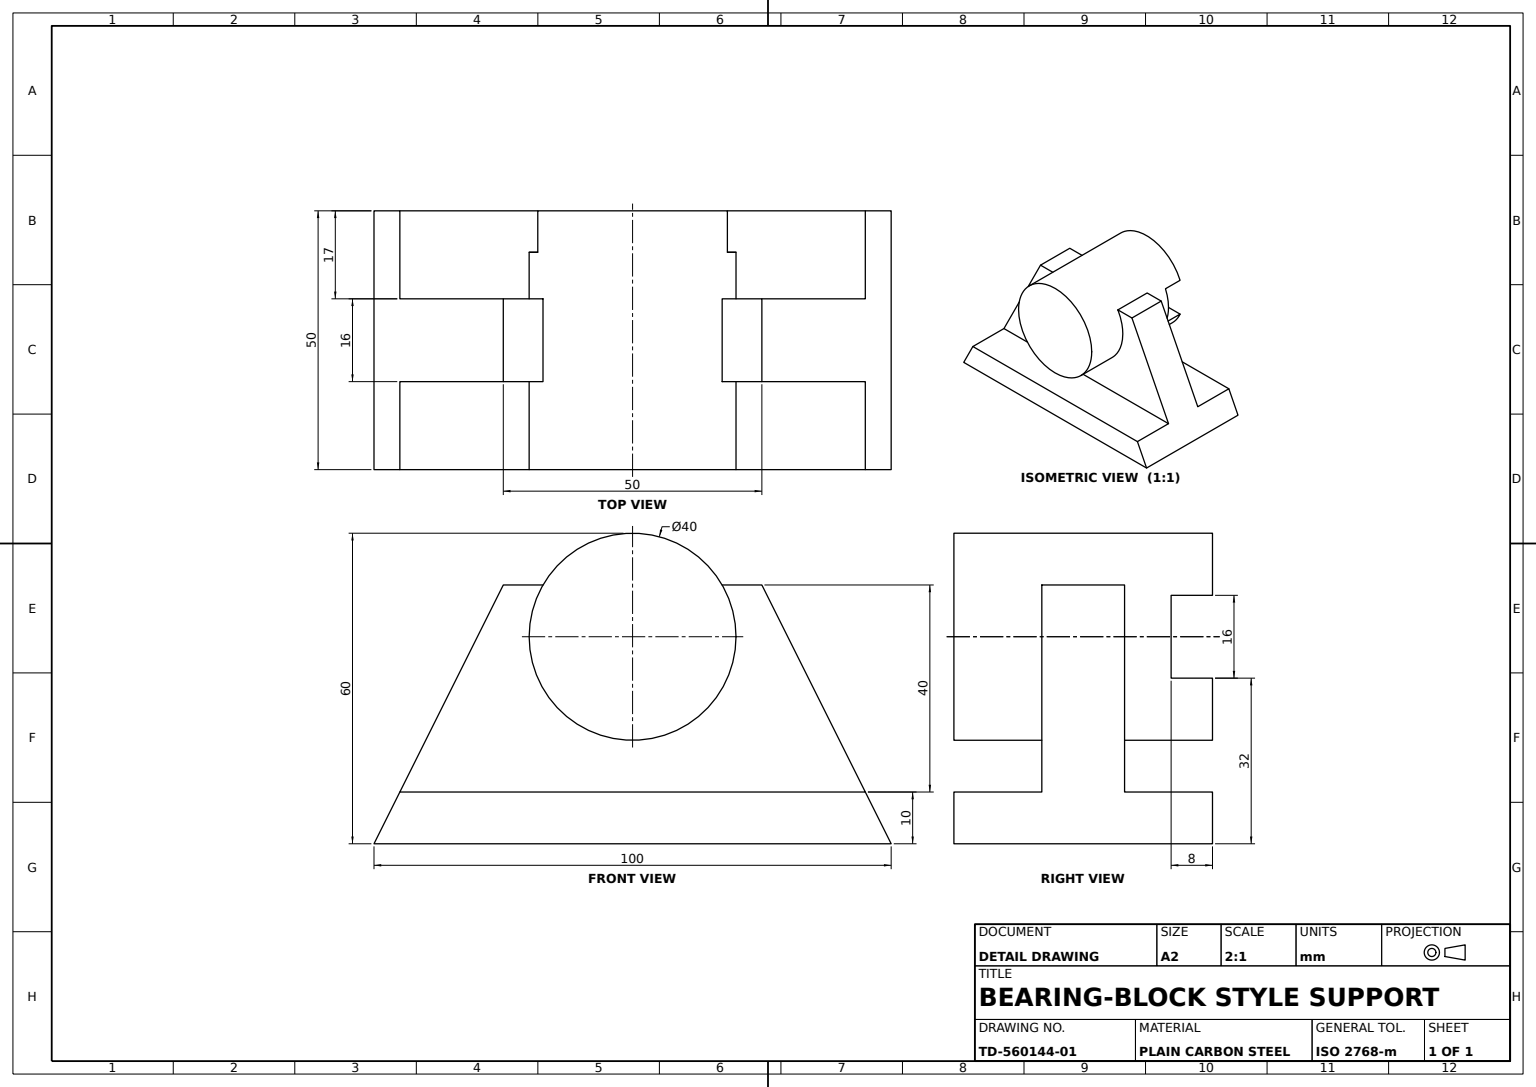
from build123d import *

# Parameters (mm, degrees)
BASE_PLATE_DEPTH        = 25
SUPPORT_UPRIGHT_DEPTH   = 8
SHAFT_CYLINDER_SKETCH_R = 20
SHAFT_CYLINDER_40_DEPTH = 25
SHAFT_START             = -8
SHAFT_END_NOTCH_DEPTH   = 8


with BuildPart() as part:
    # Base Plate Sketch → Base Plate (new, symmetric)
    with BuildSketch(Plane.XY):
        Polygon((0, 0), (100, 0), (95, 10), (5, 10), align=None)
    extrude(amount=BASE_PLATE_DEPTH, both=True)

    # Support Upright Sketch → Support Upright (add, symmetric)
    with BuildSketch(Plane.XY):
        Polygon((5, 10), (95, 10), (75, 50), (25, 50), align=None)
    extrude(amount=SUPPORT_UPRIGHT_DEPTH, both=True)

    # Shaft Cylinder Sketch → Shaft Cylinder Ø40 (add, symmetric)
    with BuildSketch(Plane.XY):
        with Locations((50, 40)):
            Circle(SHAFT_CYLINDER_SKETCH_R)
    extrude(amount=SHAFT_CYLINDER_40_DEPTH, both=True)

    # Shaft End Notch Sketch → Shaft End Notch (cut)
    with BuildSketch(Plane(origin=(0, 0, -25), x_dir=(-1, 0, 0), z_dir=(0, 0, -1)).offset(SHAFT_START)):
        with BuildLine():
            Line((-31.66969722, 48), (-68.33030278, 48))
            ThreePointArc((-68.33030278, 48), (-70, 40), (-68.33030278, 32))
            Line((-68.33030278, 32), (-31.66969722, 32))
            ThreePointArc((-31.66969722, 32), (-30, 40), (-31.66969722, 48))
        make_face()
    extrude(amount=SHAFT_END_NOTCH_DEPTH, mode=Mode.SUBTRACT)


solid = part.part
